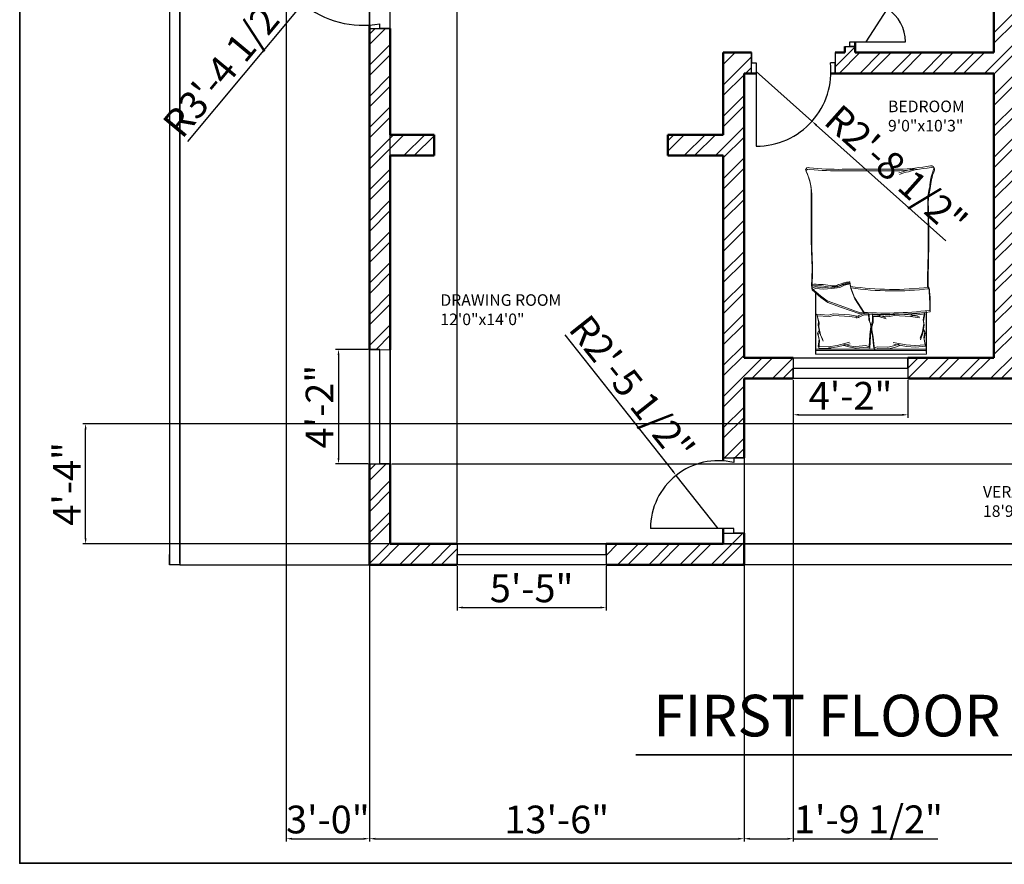
# Model space of a CAD drawing. Units: inches. Extents: x 1990 to 2869, y 1755 to 2533.
# Tile 1 of 6: x 1990 to 2415, y 1755 to 2120. Entities that reach past the tile are written whole.
import ezdxf

# ---------------------------------------------------------------- set-up
doc = ezdxf.new("R2010")
doc.units = ezdxf.units.IN
for name, color, linetype, lineweight in [('A-ANNO-DIMS', 171, 'Continuous', 18), ('A-ANNO-TTLB', 7, 'Continuous', 35), ('A-AREA-IDEN', 7, 'Continuous', 18), ('A-DOOR', 11, 'Continuous', 25), ('A-FLOR', 7, 'Continuous', 25), ('A-FURN', 8, 'Continuous', 18), ('A-GLAZ', 121, 'Continuous', 25), ('A-WALL', 7, 'Continuous', 50), ('A-WALL-SITE', 7, 'Continuous', 30)]:
    doc.layers.add(name, color=color, linetype=linetype, lineweight=lineweight)
doc.layers.add('A-WALL-PATT', color=215, linetype='Continuous', lineweight=13, true_color=0xa953a0)
doc.styles.get("Standard").update_dxf_attribs({"font": 'arial.ttf'})
doc.dimstyles.new('ISO-25', dxfattribs={"dimtxt": 12, "dimasz": 2.5, "dimexe": 1.25, "dimexo": 0.625, "dimtad": 1, "dimdec": 0, "dimlunit": 3, "dimtxsty": 'Standard', "dimcen": 2.5, "dimadec": 0, "dimazin": 0, "dimtfac": 1, "dimtdec": 0, "dimtmove": 0, "dimatfit": 3, "dimfxl": 1, "dimarcsym": 0})

# ---------------------------------------------------------------- blocks, each defined once
blk = doc.blocks.new('*D5')
at = {"layer": 'A-ANNO-DIMS', "color": 0, "lineweight": -2, "transparency": 16777216}
for p, q in [((2140.35, 1977.7), (2126.32, 1977.7)), ((2127.57, 1975.2), (2127.57, 1930.7)), ((2140.35, 1928.2), (2126.32, 1928.2))]:
    blk.add_line(p, q, dxfattribs=at)
at = {"layer": 'A-ANNO-DIMS', "color": 0, "transparency": 16777216}
for points in [[(2127.16, 1975.2), (2127.99, 1975.2), (2127.57, 1977.7)], [(2127.16, 1930.7), (2127.99, 1930.7), (2127.57, 1928.2)]]:
    blk.add_solid(points, dxfattribs=at)
at = {"layer": 'Defpoints', "color": 0, "transparency": 16777216}
for p in [(2140.97, 1977.7), (2127.57, 1928.2), (2140.97, 1928.2)]:
    blk.add_point(p, dxfattribs=at)
at = {"layer": 'A-ANNO-DIMS', "color": 0, "transparency": 16777216, "insert": (2120.92, 1952.95), "char_height": 12, "attachment_point": 5, "rotation": 90}
blk.add_mtext('4\'-2"', dxfattribs=at)
blk = doc.blocks.new('*D6')
at = {"layer": 'A-ANNO-DIMS', "color": 0, "lineweight": -2, "transparency": 16777216}
for p, q in [((2178.84, 1883.93), (2178.84, 1864.81)), ((2243.34, 1883.93), (2243.34, 1864.81)), ((2181.34, 1866.06), (2240.84, 1866.06))]:
    blk.add_line(p, q, dxfattribs=at)
at = {"layer": 'A-ANNO-DIMS', "color": 0, "transparency": 16777216}
for points in [[(2181.34, 1866.48), (2181.34, 1865.64), (2178.84, 1866.06)], [(2240.84, 1866.48), (2240.84, 1865.64), (2243.34, 1866.06)]]:
    blk.add_solid(points, dxfattribs=at)
at = {"layer": 'Defpoints', "color": 0, "transparency": 16777216}
for p in [(2178.84, 1884.55), (2243.34, 1884.55), (2243.34, 1866.06)]:
    blk.add_point(p, dxfattribs=at)
at = {"layer": 'A-ANNO-DIMS', "color": 0, "transparency": 16777216, "insert": (2211.09, 1872.79), "char_height": 12, "attachment_point": 5}
blk.add_mtext('5\'-5"', dxfattribs=at)
blk = doc.blocks.new('*D7')
at = {"layer": 'A-ANNO-DIMS', "color": 0, "lineweight": -2, "transparency": 16777216}
for p, q in [((2324.23, 1964.43), (2324.23, 1948.16)), ((2373.73, 1964.43), (2373.73, 1948.16)), ((2326.73, 1949.41), (2371.23, 1949.41))]:
    blk.add_line(p, q, dxfattribs=at)
at = {"layer": 'A-ANNO-DIMS', "color": 0, "transparency": 16777216}
for points in [[(2326.73, 1949.82), (2326.73, 1948.99), (2324.23, 1949.41)], [(2371.23, 1949.82), (2371.23, 1948.99), (2373.73, 1949.41)]]:
    blk.add_solid(points, dxfattribs=at)
at = {"layer": 'Defpoints', "color": 0, "transparency": 16777216}
for p in [(2324.23, 1965.05), (2373.73, 1965.05), (2373.73, 1949.41)]:
    blk.add_point(p, dxfattribs=at)
at = {"layer": 'A-ANNO-DIMS', "color": 0, "transparency": 16777216, "insert": (2348.98, 1956.06), "char_height": 12, "attachment_point": 5}
blk.add_mtext('4\'-2"', dxfattribs=at)
blk = doc.blocks.new('BED-DOUBLE')
for p, q in [((3.47, 63.33), (3.47, 81.44)), ((3.47, 81.44), (51.49, 81.44)), ((3.48, 63.33), (3.48, 81.44)), ((51.27, 81.44), (51.27, 54.83)), ((51.27, 81.44), (51.27, 54.83)), ((51.49, 81.44), (51.49, 80.8)), ((3.47, 79.91), (51.27, 79.91)), ((3.48, 79.91), (51.27, 79.91)), ((3.7, 62.69), (3.7, 80.8)), ((3.7, 62.69), (3.7, 80.8)), ((3.7, 79.27), (51.49, 79.27)), ((3.7, 79.27), (51.49, 79.27)), ((3.89, 78.13), (4.47, 74.95)), ((3.89, 78.13), (4.47, 74.95)), ((3.9, 78.11), (8.18, 78.43)), ((3.9, 78.11), (8.18, 78.43)), ((4.12, 77.49), (4.7, 74.31)), ((4.12, 77.49), (4.7, 74.31)), ((4.13, 77.47), (8.41, 77.8)), ((4.13, 77.47), (8.41, 77.8)), ((8.18, 78.43), (8.28, 78.42)), ((8.18, 78.43), (8.28, 78.42)), ((8.28, 78.42), (12.11, 78.13)), ((8.28, 78.42), (12.11, 78.13)), ((8.41, 77.8), (8.51, 77.78)), ((8.41, 77.8), (8.51, 77.78)), ((8.51, 77.78), (12.34, 77.49)), ((8.51, 77.78), (12.34, 77.49)), ((12.11, 78.13), (17.6, 77.11)), ((12.11, 78.13), (17.6, 77.11)), ((12.34, 77.49), (17.83, 76.48)), ((12.34, 77.49), (17.83, 76.48)), ((14.85, 77.69), (16.88, 78.42)), ((14.85, 77.69), (16.88, 78.42)), ((15.08, 77.05), (17.11, 77.78)), ((15.08, 77.05), (17.11, 77.78)), ((16.88, 78.42), (19.77, 79.14)), ((16.88, 78.42), (19.77, 79.14)), ((17.11, 77.78), (20, 78.5)), ((17.11, 77.78), (20, 78.5)), ((19.77, 79.14), (20.09, 79.14)), ((19.77, 79.14), (20.09, 79.14)), ((20, 78.5), (20.32, 78.5)), ((20, 78.5), (20.32, 78.5)), ((20.09, 79.14), (24.54, 78.99)), ((20.09, 79.14), (24.54, 78.99)), ((20.32, 78.5), (24.77, 78.36)), ((20.32, 78.5), (24.77, 78.36)), ((24.54, 78.99), (25.98, 79.57)), ((24.54, 78.99), (25.98, 79.57)), ((24.77, 78.36), (26.21, 78.93)), ((24.77, 78.36), (26.21, 78.93)), ((25.98, 79.57), (26.56, 74.22)), ((25.98, 79.57), (26.56, 74.22)), ((26.21, 78.93), (26.79, 73.58)), ((26.21, 78.93), (26.79, 73.58)), ((27.98, 78.95), (27.73, 73.58)), ((27.98, 78.95), (27.73, 73.58)), ((28.21, 78.31), (27.96, 72.94)), ((28.2, 78.31), (27.96, 72.94)), ((29.46, 78.46), (27.98, 78.95)), ((29.46, 78.46), (27.98, 78.95)), ((29.68, 77.82), (28.2, 78.31)), ((29.68, 77.82), (28.21, 78.31)), ((33.88, 78.89), (29.46, 78.46)), ((33.88, 78.89), (29.46, 78.46)), ((34.11, 78.25), (29.68, 77.82)), ((34.11, 78.25), (29.68, 77.82)), ((34.2, 78.91), (33.88, 78.89)), ((34.2, 78.91), (33.88, 78.89)), ((34.43, 78.27), (34.11, 78.25)), ((34.43, 78.27), (34.11, 78.25)), ((37.14, 78.36), (34.2, 78.91)), ((37.13, 78.36), (34.2, 78.91)), ((37.36, 77.73), (34.43, 78.27)), ((37.36, 77.73), (34.43, 78.27)), ((41.91, 78.37), (36.49, 77.02)), ((41.91, 78.37), (36.49, 77.02)), ((42.14, 77.73), (36.72, 76.38)), ((42.14, 77.73), (36.72, 76.38)), ((39.2, 77.77), (37.13, 78.36)), ((39.2, 77.77), (37.14, 78.36)), ((39.43, 77.13), (37.36, 77.73)), ((39.43, 77.13), (37.36, 77.73)), ((45.71, 78.9), (41.91, 78.37)), ((45.71, 78.9), (41.91, 78.37)), ((45.94, 78.26), (42.14, 77.73)), ((45.94, 78.26), (42.14, 77.73)), ((50.11, 78.89), (44.71, 78.98)), ((44.71, 78.98), (45.71, 78.9)), ((50.11, 78.89), (44.71, 78.98)), ((44.71, 78.98), (45.71, 78.9)), ((50.34, 78.25), (44.94, 78.34)), ((44.94, 78.34), (45.94, 78.26)), ((50.34, 78.25), (44.94, 78.34)), ((44.94, 78.34), (45.94, 78.26)), ((50.11, 78.89), (49.73, 75.68)), ((50.11, 78.89), (49.73, 75.68)), ((50.34, 78.25), (49.96, 75.04)), ((50.34, 78.25), (49.96, 75.04)), ((51.49, 80.8), (51.49, 54.19)), ((51.49, 80.8), (51.49, 54.19)), ((4.47, 74.95), (4.04, 72.34)), ((4.47, 74.95), (4.04, 72.34)), ((4.7, 74.31), (4.27, 71.7)), ((4.7, 74.31), (4.27, 71.7)), ((4.47, 68.87), (5.05, 72.49)), ((4.47, 68.87), (5.05, 72.49)), ((5.05, 72.49), (6.06, 75.24)), ((5.05, 72.49), (6.06, 75.24)), ((5.28, 71.85), (6.29, 74.6)), ((5.28, 71.85), (6.29, 74.6)), ((26.56, 74.22), (27.14, 71.04)), ((26.56, 74.22), (27.14, 71.04)), ((26.79, 73.58), (27.37, 70.4)), ((26.79, 73.58), (27.37, 70.4)), ((27.73, 73.58), (27.35, 70.37)), ((27.73, 73.58), (27.35, 70.37)), ((27.96, 72.94), (27.58, 69.73)), ((27.96, 72.94), (27.58, 69.73)), ((49.31, 73.19), (48.13, 75.86)), ((49.31, 73.19), (48.13, 75.86)), ((49.54, 72.55), (48.36, 75.23)), ((49.54, 72.55), (48.36, 75.23)), ((50.11, 69.61), (49.31, 73.19)), ((50.11, 69.61), (49.31, 73.19)), ((50.34, 68.98), (49.54, 72.55)), ((50.34, 68.98), (49.54, 72.55)), ((49.73, 75.68), (50.33, 73.1)), ((49.73, 75.68), (50.33, 73.1)), ((50.33, 73.1), (49.81, 72.06)), ((50.33, 73.1), (49.81, 72.06)), ((49.96, 75.04), (50.56, 72.47)), ((49.96, 75.04), (50.56, 72.47)), ((50.56, 72.47), (50.04, 71.42)), ((50.56, 72.47), (50.04, 71.42)), ((4.04, 72.34), (4.62, 71.33)), ((4.04, 72.34), (4.62, 71.33)), ((4.27, 71.7), (4.85, 70.69)), ((4.27, 71.7), (4.85, 70.69)), ((4.76, 67.28), (4.47, 68.87)), ((4.76, 67.28), (4.47, 68.87)), ((4.7, 68.23), (5.28, 71.85)), ((4.7, 68.23), (5.28, 71.85)), ((4.99, 66.64), (4.7, 68.23)), ((4.99, 66.64), (4.7, 68.23)), ((27.14, 69.74), (26.56, 67.86)), ((27.14, 69.74), (26.56, 67.86)), ((27.37, 69.1), (26.79, 67.22)), ((27.37, 69.1), (26.79, 67.22)), ((27.14, 71.04), (27.14, 69.74)), ((27.14, 71.04), (27.14, 69.74)), ((27.35, 70.37), (27.44, 69.07)), ((27.35, 70.37), (27.44, 69.07)), ((27.37, 70.4), (27.37, 69.1)), ((27.37, 70.4), (27.37, 69.1)), ((27.44, 69.07), (28.13, 67.23)), ((27.44, 69.07), (28.13, 67.23)), ((27.58, 69.73), (27.66, 68.43)), ((27.58, 69.73), (27.66, 68.43)), ((27.66, 68.43), (28.36, 66.59)), ((27.66, 68.43), (28.36, 66.59)), ((49.92, 68.01), (50.11, 69.61)), ((49.92, 68.01), (50.11, 69.61)), ((50.15, 67.37), (50.34, 68.98)), ((50.15, 67.37), (50.34, 68.98)), ((4.18, 64.1), (4.76, 67.28)), ((4.18, 64.1), (4.76, 67.28)), ((9.28, 64.82), (4.18, 64.1)), ((9.28, 64.82), (4.18, 64.1)), ((4.41, 63.46), (4.99, 66.64)), ((4.41, 63.46), (4.99, 66.64)), ((9.51, 64.19), (4.41, 63.46)), ((9.51, 64.19), (4.41, 63.46)), ((6.38, 65.81), (10.41, 65.15)), ((6.38, 65.81), (10.41, 65.15)), ((6.61, 65.18), (10.64, 64.51)), ((6.61, 65.18), (10.64, 64.51)), ((10.41, 65.15), (9.28, 64.82)), ((10.41, 65.15), (9.28, 64.82)), ((10.64, 64.51), (9.51, 64.19)), ((10.64, 64.51), (9.51, 64.19)), ((10.41, 65.15), (17.42, 64.72)), ((10.41, 65.15), (17.42, 64.72)), ((10.64, 64.51), (17.65, 64.08)), ((10.64, 64.51), (17.65, 64.08)), ((17.42, 64.72), (19.38, 65.27)), ((17.42, 64.72), (19.38, 65.27)), ((17.65, 64.08), (19.61, 64.63)), ((17.65, 64.08), (19.61, 64.63)), ((19.38, 65.27), (24.52, 64.87)), ((19.38, 65.27), (24.52, 64.87)), ((19.61, 64.63), (24.74, 64.23)), ((19.61, 64.63), (24.74, 64.23)), ((24.1, 65.18), (20.96, 66.27)), ((24.1, 65.18), (20.96, 66.27)), ((24.33, 64.54), (21.19, 65.63)), ((24.33, 64.54), (21.19, 65.63)), ((26.56, 65.18), (24.1, 65.18)), ((26.56, 65.18), (24.1, 65.18)), ((26.79, 64.54), (24.33, 64.54)), ((26.79, 64.54), (24.33, 64.54)), ((26.56, 67.86), (26.56, 65.18)), ((26.56, 67.86), (26.56, 65.18)), ((26.79, 67.22), (26.79, 64.54)), ((26.79, 67.22), (26.79, 64.54)), ((28.13, 67.23), (28.3, 64.55)), ((28.13, 67.23), (28.3, 64.55)), ((28.3, 64.55), (30.75, 64.7)), ((28.3, 64.55), (30.75, 64.7)), ((28.36, 66.59), (28.53, 63.91)), ((28.36, 66.59), (28.53, 63.91)), ((28.53, 63.91), (30.98, 64.06)), ((28.53, 63.91), (30.98, 64.06)), ((30.26, 64.06), (34.45, 57.57)), ((30.26, 64.06), (34.45, 57.57)), ((30.75, 64.7), (33.82, 65.99)), ((30.75, 64.7), (33.82, 65.99)), ((30.98, 64.06), (34.05, 65.35)), ((30.98, 64.06), (34.05, 65.35)), ((40.64, 61.13), (32.31, 64.06)), ((40.64, 61.13), (32.31, 64.06)), ((32.56, 65.81), (36.6, 65.15)), ((32.56, 65.81), (36.6, 65.15)), ((32.79, 65.18), (36.82, 64.51)), ((32.79, 65.18), (36.82, 64.51)), ((36.6, 65.15), (43.61, 64.72)), ((36.6, 65.15), (43.61, 64.72)), ((36.82, 64.51), (43.83, 64.08)), ((36.82, 64.51), (43.83, 64.08)), ((43.61, 64.72), (45.57, 65.27)), ((43.61, 64.72), (45.57, 65.27)), ((43.83, 64.08), (45.79, 64.63)), ((43.83, 64.08), (45.79, 64.63)), ((45.57, 65.27), (50.7, 64.87)), ((45.57, 65.27), (50.7, 64.87)), ((45.79, 64.63), (50.93, 64.23)), ((45.79, 64.63), (50.93, 64.23)), ((50.7, 64.87), (49.92, 68.01)), ((50.7, 64.87), (49.92, 68.01)), ((50.93, 64.23), (50.15, 67.37)), ((50.93, 64.23), (50.15, 67.37)), ((30.49, 63.42), (34.68, 56.93)), ((30.49, 63.42), (34.68, 56.93)), ((40.87, 60.49), (32.53, 63.42)), ((40.87, 60.49), (32.53, 63.42)), ((46.22, 59.11), (40.64, 61.13)), ((46.22, 59.11), (40.64, 61.13)), ((46.45, 58.48), (40.87, 60.49)), ((46.45, 58.48), (40.87, 60.49)), ((34.45, 57.57), (36.15, 53.08)), ((34.45, 57.57), (36.15, 53.08)), ((34.68, 56.93), (36.38, 52.44)), ((34.68, 56.93), (36.38, 52.44)), ((49.16, 56.95), (46.22, 59.11)), ((49.16, 56.95), (46.22, 59.11)), ((49.39, 56.31), (46.45, 58.48)), ((49.39, 56.31), (46.45, 58.48)), ((52.87, 53.7), (49.16, 56.95)), ((52.87, 53.7), (49.16, 56.95)), ((53.1, 53.06), (49.39, 56.31)), ((53.1, 53.06), (49.39, 56.31)), ((36.15, 53.08), (36.46, 51.07)), ((36.15, 53.08), (36.46, 51.07)), ((36.38, 52.44), (36.69, 50.43)), ((36.38, 52.44), (36.69, 50.43)), ((36.46, 51.07), (38.94, 51.69)), ((36.46, 51.07), (38.94, 51.69)), ((38.94, 51.69), (40.95, 52.61)), ((38.94, 51.69), (40.95, 52.61)), ((39.17, 51.05), (41.18, 51.97)), ((39.17, 51.05), (41.18, 51.97)), ((40.95, 52.61), (44.36, 53.08)), ((40.95, 52.61), (44.36, 53.08)), ((41.18, 51.97), (44.59, 52.44)), ((41.18, 51.97), (44.59, 52.44)), ((44.36, 53.08), (48.23, 53.39)), ((44.36, 53.08), (48.23, 53.39)), ((44.59, 52.44), (48.46, 52.75)), ((44.59, 52.44), (48.46, 52.75)), ((48.23, 53.39), (51.33, 53.08)), ((48.23, 53.39), (51.33, 53.08)), ((48.46, 52.75), (51.56, 52.44)), ((48.46, 52.75), (51.56, 52.44)), ((51.33, 53.08), (52.87, 53.7)), ((51.33, 53.08), (52.87, 53.7)), ((51.56, 52.44), (53.1, 53.06)), ((51.56, 52.44), (53.1, 53.06)), ((52.95, 51.95), (52.87, 53.7, 3.87)), ((52.95, 51.95), (52.87, 53.7, 3.87)), ((53.18, 51.31), (53.1, 53.06, 3.87)), ((53.18, 51.31), (53.1, 53.06, 3.87)), ((36.69, 50.43), (39.17, 51.05)), ((36.69, 50.43), (39.17, 51.05)), ((15.06, 2.2), (39.68, 2.2)), ((15.06, 2.2), (39.68, 2.2)), ((15.29, 1.56), (39.91, 1.56)), ((15.29, 1.56), (39.91, 1.56))]:
    blk.add_line(p, q)
for centre, radius, start, end in [((21.36, -100.61), 164.97, 86.0865, 96.7821), ((21.36, -100.61), 164.97, 86.0865, 96.7821), ((85.16, 61.35), 83.31, 178.7218, 185.604), ((85.16, 61.35), 83.31, 178.7218, 185.604), ((85.39, 60.71), 83.31, 178.7218, 185.604), ((85.39, 60.71), 83.31, 178.7218, 185.604), ((21.59, -101.25), 164.97, 86.0865, 96.7821), ((21.59, -101.25), 164.97, 86.0865, 96.7821), ((17.76, -74.87), 129.02, 81.7845, 96.9006), ((17.76, -74.87), 129.02, 81.7845, 96.9006), ((17.98, -75.51), 129.02, 81.7845, 96.9006), ((17.98, -75.51), 129.02, 81.7845, 96.9006), ((-167.31, 50.27), 170.11, 358.4762, 1.0082), ((-167.31, 50.27), 170.11, 358.4762, 1.0082), ((-167.08, 49.63), 170.11, 358.4762, 1.0082), ((-167.08, 49.63), 170.11, 358.4762, 1.0082), ((31.15, 79.96), 29.65, 280.6617, 289.8806), ((31.15, 79.96), 29.65, 280.6617, 289.8806), ((31.38, 79.32), 29.65, 280.6617, 289.8806), ((31.38, 79.32), 29.65, 280.6617, 289.8806), ((43.74, 46.38), 6.22, 78.6608, 113.7384), ((43.74, 46.38), 6.22, 78.6608, 113.7384), ((43.97, 45.74), 6.22, 78.6608, 113.7384), ((43.97, 45.74), 6.22, 78.6608, 113.7384), ((51.33, 88.1), 36.18, 259.8763, 272.5657), ((51.33, 88.1), 36.18, 259.8763, 272.5657), ((51.56, 87.46), 36.18, 259.8763, 272.5657), ((51.56, 87.46), 36.18, 259.8763, 272.5657), ((182.27, 45.13), 129.5, 176.9791, 183.8365), ((182.27, 45.13), 129.5, 176.9791, 183.8365), ((182.49, 44.49), 129.5, 176.9791, 183.8365), ((182.49, 44.49), 129.5, 176.9791, 183.8365), ((36.64, 51), 0.185, 160.2464, 271.1377), ((36.64, 51), 0.185, 160.2464, 271.1377), ((36.86, 50.36), 0.185, 160.2464, 271.1377), ((36.86, 50.36), 0.185, 160.2464, 271.1377), ((484.82, 30.83), 482.31, 178.2277, 181.7185), ((484.82, 30.83), 482.31, 178.2277, 181.7185), ((485.05, 30.19), 482.31, 178.2277, 181.7185), ((485.05, 30.19), 482.31, 178.2277, 181.7185), ((-4508.74, 13.62), 4561.86, 0.00217, 0.28689), ((-4508.74, 13.62), 4561.86, 0.00217, 0.28689), ((-4508.52, 12.98), 4561.86, 0.00217, 0.28689), ((-4508.52, 12.98), 4561.86, 0.00217, 0.28689), ((-26.9, 16.93), 29.63, 346.0648, 358.9113), ((-26.9, 16.93), 29.63, 346.0648, 358.9113), ((-26.67, 16.29), 29.63, 346.0648, 358.9113), ((-26.67, 16.29), 29.63, 346.0648, 358.9113), ((76.16, 12.78), 23.07, 177.4714, 206.4681), ((76.16, 12.78), 23.07, 177.4714, 206.4681), ((76.39, 12.14), 23.07, 177.4714, 206.4681), ((76.39, 12.14), 23.07, 177.4714, 206.4681), ((-21.66, 11.17), 23.56, 337.9751, 356.652), ((-21.66, 11.17), 23.56, 337.9751, 356.652), ((-21.43, 10.53), 23.56, 337.9751, 356.652), ((-21.43, 10.53), 23.56, 337.9751, 356.652), ((1.09, 1.73), 1.09, 146.1736, 293.4781), ((1.09, 1.73), 1.09, 146.1736, 293.4781), ((1.32, 1.09), 1.09, 146.1736, 293.4781), ((1.32, 1.09), 1.09, 146.1736, 293.4781), ((21.43, -119.39), 121.76, 92.9958, 99.4091), ((21.43, -119.39), 121.76, 92.9958, 99.4091), ((21.66, -120.03), 121.76, 92.9958, 99.4091), ((21.65, -120.03), 121.76, 92.9958, 99.4091), ((-17.22, 105.15), 106.46, 283.3832, 287.7053), ((-17.22, 105.15), 106.46, 283.3832, 287.7053), ((-16.99, 104.52), 106.46, 283.3832, 287.7053), ((-16.99, 104.52), 106.46, 283.3832, 287.7053), ((41.15, -130.83), 133.04, 84.4998, 90.6351), ((41.15, -130.83), 133.04, 84.4998, 90.6351), ((41.38, -131.47), 133.04, 84.4998, 90.6351), ((41.38, -131.47), 133.04, 84.4998, 90.6351), ((54.41, 2.57), 1.1, 242.6588, 356.02), ((54.41, 2.57), 1.1, 242.6588, 356.02), ((54.64, 1.93), 1.1, 242.6588, 356.02), ((54.64, 1.93), 1.1, 242.6588, 356.02)]:
    blk.add_arc(centre, radius, start, end)
blk = doc.blocks.new('WIN-49_5IN')
for p, q in [((0, 9), (0, 0)), ((0, 9), (49.5, 9)), ((49.5, 4.5), (49.5, 9)), ((49.5, 9), (49.5, 0)), ((0, 0), (0, 4.5)), ((0, 4.5), (49.5, 4.5)), ((49.5, 0), (0, 0))]:
    blk.add_line(p, q)
blk = doc.blocks.new('WIN-64_5IN')
for p, q in [((0, 9), (0, 0)), ((0, 9), (64.5, 9)), ((64.5, 4.5), (64.5, 9)), ((64.5, 9), (64.5, 0)), ((0, 0), (0, 4.5)), ((0, 4.5), (64.5, 4.5)), ((64.5, 0), (0, 0))]:
    blk.add_line(p, q)
blk = doc.blocks.new('*D23')
at = {"layer": 'A-ANNO-DIMS', "color": 0, "lineweight": -2, "transparency": 16777216}
for p, q in [((2435.03, 2169.19), (2437.82, 2169.19)), ((2436.57, 2166.69), (2436.57, 2161.95)), ((2435.03, 2159.45), (2437.82, 2159.45)), ((2436.57, 2159.45), (2436.57, 2054.59))]:
    blk.add_line(p, q, dxfattribs=at)
at = {"layer": 'A-ANNO-DIMS', "color": 0, "transparency": 16777216}
for points in [[(2436.15, 2166.69), (2436.99, 2166.69), (2436.57, 2169.19)], [(2436.15, 2161.95), (2436.99, 2161.95), (2436.57, 2159.45)]]:
    blk.add_solid(points, dxfattribs=at)
at = {"layer": 'Defpoints', "color": 0, "transparency": 16777216}
for p in [(2434.41, 2169.19), (2434.41, 2159.45), (2436.57, 2159.45)]:
    blk.add_point(p, dxfattribs=at)
at = {"layer": 'A-ANNO-DIMS', "color": 0, "transparency": 16777216, "insert": (2429.74, 2105.77), "char_height": 12, "attachment_point": 5, "rotation": 90}
blk.add_mtext('0\'-9 1/2" TYP.', dxfattribs=at)
blk = doc.blocks.new('*D24')
at = {"layer": 'A-ANNO-DIMS', "color": 0, "lineweight": -2, "transparency": 16777216}
for p, q in [((2149.97, 1894.18), (2149.97, 2365.55)), ((2152.47, 2364.3), (2176.34, 2364.3)), ((2178.84, 1894.18), (2178.84, 2365.55)), ((2178.84, 2364.3), (2214.69, 2364.3))]:
    blk.add_line(p, q, dxfattribs=at)
at = {"layer": 'A-ANNO-DIMS', "color": 0, "transparency": 16777216}
for points in [[(2152.47, 2364.72), (2152.47, 2363.88), (2149.97, 2364.3)], [(2176.34, 2364.72), (2176.34, 2363.88), (2178.84, 2364.3)]]:
    blk.add_solid(points, dxfattribs=at)
at = {"layer": 'Defpoints', "color": 0, "transparency": 16777216}
for p in [(2178.84, 2364.3), (2149.97, 1893.55), (2178.84, 1893.55)]:
    blk.add_point(p, dxfattribs=at)
at = {"layer": 'A-ANNO-DIMS', "color": 0, "transparency": 16777216, "insert": (2198.02, 2371.05), "char_height": 12, "attachment_point": 5}
blk.add_mtext('2\'-5"', dxfattribs=at)
blk = doc.blocks.new('*D25')
at = {"layer": 'A-ANNO-DIMS', "color": 0, "lineweight": -2, "transparency": 16777216}
for p, q in [((2058.97, 1885.18), (2058.97, 2365.55)), ((2061.47, 2364.3), (2138.47, 2364.3)), ((2140.97, 1885.18), (2140.97, 2365.55))]:
    blk.add_line(p, q, dxfattribs=at)
at = {"layer": 'A-ANNO-DIMS', "color": 0, "transparency": 16777216}
for points in [[(2061.47, 2364.72), (2061.47, 2363.88), (2058.97, 2364.3)], [(2138.47, 2364.72), (2138.47, 2363.88), (2140.97, 2364.3)]]:
    blk.add_solid(points, dxfattribs=at)
at = {"layer": 'Defpoints', "color": 0, "transparency": 16777216}
for p in [(2140.97, 2364.3), (2058.97, 1884.55), (2140.97, 1884.55)]:
    blk.add_point(p, dxfattribs=at)
at = {"layer": 'A-ANNO-DIMS', "color": 0, "transparency": 16777216, "insert": (2099.97, 2371.05), "char_height": 12, "attachment_point": 5}
blk.add_mtext('6\'-10"', dxfattribs=at)
blk = doc.blocks.new('*D26')
at = {"layer": 'A-ANNO-DIMS', "color": 0, "lineweight": -2, "transparency": 16777216}
for p, q in [((2140.97, 1883.93), (2140.97, 1764.83)), ((2302.97, 1883.93), (2302.97, 1764.83)), ((2143.47, 1766.08), (2300.47, 1766.08))]:
    blk.add_line(p, q, dxfattribs=at)
at = {"layer": 'A-ANNO-DIMS', "color": 0, "transparency": 16777216}
for points in [[(2143.47, 1766.49), (2143.47, 1765.66), (2140.97, 1766.08)], [(2300.47, 1766.49), (2300.47, 1765.66), (2302.97, 1766.08)]]:
    blk.add_solid(points, dxfattribs=at)
at = {"layer": 'Defpoints', "color": 0, "transparency": 16777216}
for p in [(2140.97, 1884.55), (2302.97, 1884.55), (2302.97, 1766.08)]:
    blk.add_point(p, dxfattribs=at)
at = {"layer": 'A-ANNO-DIMS', "color": 0, "transparency": 16777216, "insert": (2221.97, 1772.83), "char_height": 12, "attachment_point": 5}
blk.add_mtext('13\'-6"', dxfattribs=at)
blk = doc.blocks.new('*D28')
at = {"layer": 'A-ANNO-DIMS', "color": 0, "lineweight": -2, "transparency": 16777216}
for p, q in [((2812.72, 1928.2), (2812.72, 2001.34)), ((2150.6, 1928.2), (2813.97, 1928.2)), ((2812.72, 1896.05), (2812.72, 1925.7)), ((2150.6, 1893.55), (2813.97, 1893.55))]:
    blk.add_line(p, q, dxfattribs=at)
at = {"layer": 'A-ANNO-DIMS', "color": 0, "transparency": 16777216}
for points in [[(2812.3, 1925.7), (2813.14, 1925.7), (2812.72, 1928.2)], [(2812.3, 1896.05), (2813.14, 1896.05), (2812.72, 1893.55)]]:
    blk.add_solid(points, dxfattribs=at)
at = {"layer": 'Defpoints', "color": 0, "transparency": 16777216}
for p in [(2149.97, 1928.2), (2812.72, 1928.2), (2149.97, 1893.55)]:
    blk.add_point(p, dxfattribs=at)
at = {"layer": 'A-ANNO-DIMS', "color": 0, "transparency": 16777216, "insert": (2805.89, 1966.02), "char_height": 12, "attachment_point": 5, "rotation": 90}
blk.add_mtext('2\'-10 1/2"', dxfattribs=at)
blk = doc.blocks.new('*D29')
at = {"layer": 'A-ANNO-DIMS', "color": 0, "lineweight": -2, "transparency": 16777216}
for p, q in [((2680.35, 1945.55), (2016.97, 1945.55)), ((2018.22, 1896.05), (2018.22, 1943.05)), ((2680.35, 1893.55), (2016.97, 1893.55))]:
    blk.add_line(p, q, dxfattribs=at)
at = {"layer": 'A-ANNO-DIMS', "color": 0, "transparency": 16777216}
for points in [[(2017.8, 1943.05), (2018.64, 1943.05), (2018.22, 1945.55)], [(2017.8, 1896.05), (2018.64, 1896.05), (2018.22, 1893.55)]]:
    blk.add_solid(points, dxfattribs=at)
at = {"layer": 'Defpoints', "color": 0, "transparency": 16777216}
for p in [(2018.22, 1945.55), (2680.97, 1945.55), (2680.97, 1893.55)]:
    blk.add_point(p, dxfattribs=at)
at = {"layer": 'A-ANNO-DIMS', "color": 0, "transparency": 16777216, "insert": (2011.6, 1919.55), "char_height": 12, "attachment_point": 5, "rotation": 90}
blk.add_mtext('4\'-4"', dxfattribs=at)
blk = doc.blocks.new('*D31')
at = {"layer": 'A-ANNO-DIMS', "color": 0, "lineweight": -2, "transparency": 16777216}
for p, q in [((2302.97, 1964.43), (2302.97, 1764.83)), ((2324.23, 1964.43), (2324.23, 1764.83)), ((2305.47, 1766.08), (2321.73, 1766.08)), ((2324.23, 1766.08), (2386.71, 1766.08))]:
    blk.add_line(p, q, dxfattribs=at)
at = {"layer": 'A-ANNO-DIMS', "color": 0, "transparency": 16777216}
for points in [[(2305.47, 1766.49), (2305.47, 1765.66), (2302.97, 1766.08)], [(2321.73, 1766.49), (2321.73, 1765.66), (2324.23, 1766.08)]]:
    blk.add_solid(points, dxfattribs=at)
at = {"layer": 'Defpoints', "color": 0, "transparency": 16777216}
for p in [(2302.97, 1965.05), (2324.23, 1965.05), (2324.23, 1766.08)]:
    blk.add_point(p, dxfattribs=at)
at = {"layer": 'A-ANNO-DIMS', "color": 0, "transparency": 16777216, "insert": (2356.72, 1772.91), "char_height": 12, "attachment_point": 5}
blk.add_mtext('1\'-9 1/2"', dxfattribs=at)
blk = doc.blocks.new('*D33')
at = {"layer": 'A-ANNO-DIMS', "color": 0, "lineweight": -2, "transparency": 16777216}
for p, q in [((2104.97, 2165.93), (2104.97, 1764.83)), ((2140.97, 2165.93), (2140.97, 1764.83)), ((2107.47, 1766.08), (2138.47, 1766.08))]:
    blk.add_line(p, q, dxfattribs=at)
at = {"layer": 'A-ANNO-DIMS', "color": 0, "transparency": 16777216}
for points in [[(2107.47, 1766.49), (2107.47, 1765.66), (2104.97, 1766.08)], [(2138.47, 1766.49), (2138.47, 1765.66), (2140.97, 1766.08)]]:
    blk.add_solid(points, dxfattribs=at)
at = {"layer": 'Defpoints', "color": 0, "transparency": 16777216}
for p in [(2104.97, 2166.55), (2140.97, 2166.55), (2140.97, 1766.08)]:
    blk.add_point(p, dxfattribs=at)
at = {"layer": 'A-ANNO-DIMS', "color": 0, "transparency": 16777216, "insert": (2122.97, 1772.83), "char_height": 12, "attachment_point": 5}
blk.add_mtext('3\'-0"', dxfattribs=at)
blk = doc.blocks.new('*D50')
at = {"layer": 'A-ANNO-DIMS', "color": 0, "lineweight": -2, "transparency": 16777216}
for p, q in [((2138.1, 2158.48), (2112.11, 2127.26)), ((2062.46, 2067.62), (2110.51, 2125.33))]:
    blk.add_line(p, q, dxfattribs=at)
at = {"layer": 'A-ANNO-DIMS', "color": 0, "transparency": 16777216}
blk.add_solid([(2110.19, 2125.6), (2110.83, 2125.07), (2112.11, 2127.26)], dxfattribs=at)
at = {"layer": 'Defpoints', "color": 0, "transparency": 16777216}
for p in [(2138.1, 2158.48), (2112.11, 2127.26)]:
    blk.add_point(p, dxfattribs=at)
at = {"layer": 'A-ANNO-DIMS', "color": 0, "transparency": 16777216, "insert": (2080.43, 2099.89), "char_height": 12, "attachment_point": 5, "rotation": 50.2228}
blk.add_mtext('R3\'-4 1/2"', dxfattribs=at)
blk = doc.blocks.new('*D52')
at = {"layer": 'A-ANNO-DIMS', "color": 0, "lineweight": -2, "transparency": 16777216}
for p, q in [((2225.37, 1984.01), (2272.02, 1925.17)), ((2291.79, 1900.24), (2273.57, 1923.21))]:
    blk.add_line(p, q, dxfattribs=at)
at = {"layer": 'A-ANNO-DIMS', "color": 0, "transparency": 16777216}
blk.add_solid([(2272.35, 1925.43), (2271.69, 1924.91), (2273.57, 1923.21)], dxfattribs=at)
at = {"layer": 'Defpoints', "color": 0, "transparency": 16777216}
for p in [(2273.57, 1923.21), (2291.79, 1900.24)]:
    blk.add_point(p, dxfattribs=at)
at = {"layer": 'A-ANNO-DIMS', "color": 0, "transparency": 16777216, "insert": (2253.27, 1959.81), "char_height": 12, "attachment_point": 5, "rotation": 308.4096}
blk.add_mtext('R2\'-5 1/2"', dxfattribs=at)
blk = doc.blocks.new('*D57')
at = {"layer": 'A-ANNO-DIMS', "color": 0, "lineweight": -2, "transparency": 16777216}
for p, q in [((2308.2, 2097.87), (2332.31, 2076.36)), ((2390.23, 2024.71), (2334.18, 2074.69))]:
    blk.add_line(p, q, dxfattribs=at)
at = {"layer": 'A-ANNO-DIMS', "color": 0, "transparency": 16777216}
blk.add_solid([(2334.46, 2075.01), (2333.9, 2074.38), (2332.31, 2076.36)], dxfattribs=at)
at = {"layer": 'Defpoints', "color": 0, "transparency": 16777216}
for p in [(2308.2, 2097.87), (2332.31, 2076.36)]:
    blk.add_point(p, dxfattribs=at)
at = {"layer": 'A-ANNO-DIMS', "color": 0, "transparency": 16777216, "insert": (2367.68, 2053.97), "char_height": 12, "attachment_point": 5, "rotation": 318.2723}
blk.add_mtext('R2\'-8 1/2"', dxfattribs=at)
blk = doc.blocks.new('*D61')
at = {"layer": 'A-ANNO-DIMS', "color": 0, "lineweight": -2, "transparency": 16777216}
for p, q in [((2391.86, 2166.71), (2366.3, 2127.11)), ((2355.72, 2110.72), (2364.94, 2125.01))]:
    blk.add_line(p, q, dxfattribs=at)
at = {"layer": 'A-ANNO-DIMS', "color": 0, "transparency": 16777216}
blk.add_solid([(2365.95, 2127.34), (2366.65, 2126.88), (2364.94, 2125.01)], dxfattribs=at)
at = {"layer": 'Defpoints', "color": 0, "transparency": 16777216}
for p in [(2364.94, 2125.01), (2355.72, 2110.72)]:
    blk.add_point(p, dxfattribs=at)
at = {"layer": 'A-ANNO-DIMS', "color": 0, "transparency": 16777216, "insert": (2374.09, 2151.62), "char_height": 12, "attachment_point": 5, "rotation": 57.1524}
blk.add_mtext('R1\'-5"', dxfattribs=at)

msp = doc.modelspace()

# ---------------------------------------------------------------- hatches: boundary and pattern name
at = {"layer": 'A-WALL-PATT'}
h = msp.add_hatch(dxfattribs=at)
h.set_pattern_fill('ANSI32', color=256)
h.paths.add_polyline_path([(2193.46, 2287.55), (2131.97, 2287.55), (2131.97, 2278.55), (2193.46, 2278.55)])
h.paths.add_polyline_path([(2113.97, 2278.55), (2113.97, 2287.55), (2104.97, 2287.55), (2104.97, 2257.5), (2113.97, 2257.5)])
h.paths.add_polyline_path([(2113.97, 2205), (2104.97, 2205), (2104.97, 2166.55), (2140.97, 2166.55), (2140.97, 2160.48), (2149.97, 2160.48), (2149.97, 2166.55), (2170.14, 2166.55), (2170.14, 2175.55), (2113.97, 2175.55)])
h.paths.add_polyline_path([(2278.97, 2287.55), (2244.47, 2287.55), (2244.47, 2278.55), (2274.47, 2278.55), (2274.47, 2200.55), (2226.47, 2200.55), (2226.47, 2219.37), (2221.97, 2219.37), (2221.97, 2175.55), (2221.97, 2166.55), (2226.47, 2166.55), (2226.47, 2196.05), (2274.47, 2196.05), (2274.47, 2166.55), (2284.01, 2166.55), (2284.01, 2171.05), (2284.01, 2175.55), (2278.97, 2175.55), (2278.97, 2278.55)])
h.paths.add_polyline_path([(2226.47, 2283.05), (2226.47, 2287.55), (2217.66, 2287.55), (2217.66, 2283.05), (2217.66, 2278.55), (2221.97, 2278.55), (2221.97, 2255.21), (2226.47, 2255.21), (2226.47, 2278.55)])
h.paths.add_polyline_path([(2560.97, 2328.05), (2551.97, 2328.05), (2269.97, 2328.05), (2269.97, 2319.05), (2278.97, 2319.05), (2410.97, 2319.05), (2410.97, 2187.05), (2346.47, 2187.05), (2346.47, 2175.55), (2319.77, 2175.55), (2319.77, 2166.55), (2346.47, 2166.55), (2346.47, 2128.22), (2350.97, 2128.22), (2350.97, 2178.05), (2410.97, 2178.05), (2410.97, 2175.55), (2410.97, 2106.05), (2350.97, 2106.05), (2350.97, 2108.72), (2348.72, 2108.72), (2346.47, 2108.72), (2346.47, 2106.05), (2342.3, 2106.05), (2342.3, 2097.05), (2346.47, 2097.05), (2350.97, 2097.05), (2410.97, 2097.05), (2410.97, 1974.05), (2373.73, 1974.05), (2373.73, 1965.05), (2419.97, 1965.05), (2447.99, 1965.05), (2447.99, 1969.55), (2447.99, 1974.05), (2419.97, 1974.05), (2419.97, 2097.05), (2484.47, 2097.05), (2489.55, 2097.05), (2489.55, 2106.05), (2484.47, 2106.05), (2484.47, 2108.84), (2482.22, 2108.84), (2479.97, 2108.84), (2479.97, 2106.05), (2419.97, 2106.05), (2419.97, 2175.55), (2419.97, 2178.05), (2479.97, 2178.05), (2479.97, 2128.49), (2484.47, 2128.49), (2484.47, 2166.55), (2511.88, 2166.55), (2511.88, 2171.05), (2511.88, 2175.55), (2484.47, 2175.55), (2484.47, 2187.05), (2479.97, 2187.05), (2419.97, 2187.05), (2419.97, 2319.05), (2551.97, 2319.05), (2560.97, 2319.05)])
h.paths.add_polyline_path([(2586.47, 2292.05), (2560.97, 2292.05), (2551.97, 2292.05), (2551.97, 2175.55), (2547.37, 2175.55), (2547.37, 2166.55), (2556.47, 2166.55), (2556.47, 2175.55), (2556.47, 2205.05), (2604.47, 2205.05), (2604.47, 2166.55), (2608.97, 2166.55), (2608.97, 2175.55), (2608.97, 2205.05), (2608.97, 2228.1), (2604.47, 2228.1), (2604.47, 2209.55), (2556.47, 2209.55), (2556.47, 2283.05), (2586.47, 2283.05)])
h.paths.add_polyline_path([(2691.55, 2292.05), (2690.86, 2292.05), (2636.82, 2292.05), (2636.82, 2283.05), (2691.55, 2283.05)])
h.paths.add_polyline_path([(2725.97, 2292.05), (2716.97, 2292.05), (2709.55, 2292.05), (2709.55, 2287.55), (2709.55, 2283.05), (2716.97, 2283.05), (2716.97, 2263.68), (2725.97, 2263.68)])
h.paths.add_polyline_path([(2725.97, 2199.18), (2716.97, 2199.18), (2716.97, 2180.05), (2716.97, 2175.55), (2650.43, 2175.55), (2650.43, 2166.55), (2680.97, 2166.55), (2680.97, 2159.77), (2689.97, 2159.77), (2689.97, 2166.55), (2725.97, 2166.55)])
h.paths.add_polyline_path([(2536.97, 2061.55), (2554.82, 2061.55), (2554.82, 2070.55), (2536.97, 2070.55), (2536.97, 2097.05), (2536.97, 2106.05), (2524.42, 2106.05), (2524.42, 2101.55), (2524.42, 2097.05), (2527.97, 2097.05), (2527.97, 1974.05), (2497.49, 1974.05), (2497.49, 1965.05), (2527.97, 1965.05), (2527.97, 1929.96), (2536.97, 1929.96)])
h.paths.add_polyline_path([(2689.97, 1945.55), (2685.47, 1945.55), (2680.97, 1945.55), (2680.97, 1893.55), (2625.68, 1893.55), (2625.68, 1884.55), (2689.97, 1884.55), (2689.97, 1893.55)])
h.paths.add_polyline_path([(2168.89, 2070.55), (2149.97, 2070.55), (2149.97, 2116.52), (2145.47, 2116.52), (2140.97, 2116.52), (2140.97, 1977.7), (2145.47, 1977.7), (2145.47, 1977.63), (2149.97, 1977.55), (2149.97, 2061.55), (2168.89, 2061.55)])
h.paths.add_polyline_path([(2302.97, 2097.05), (2306.2, 2097.05), (2306.2, 2106.05), (2293.97, 2106.05), (2293.97, 2097.05), (2293.97, 2070.55), (2269.93, 2070.55), (2269.93, 2061.55), (2293.97, 2061.55), (2293.97, 1930.78), (2302.97, 1930.78), (2302.97, 1965.05), (2324.23, 1965.05), (2324.23, 1969.55), (2324.23, 1974.05), (2302.97, 1974.05)])
h.paths.add_polyline_path([(2149.97, 1928.2), (2145.47, 1928.2), (2140.97, 1928.2), (2140.97, 1889.05), (2140.97, 1884.55), (2178.84, 1884.55), (2178.84, 1889.05), (2178.84, 1893.55), (2149.97, 1893.55)])
h.paths.add_polyline_path([(2302.97, 1898.24), (2298.47, 1898.24), (2293.97, 1898.24), (2293.97, 1893.55), (2243.34, 1893.55), (2243.34, 1884.55), (2302.97, 1884.55)])

# ---------------------------------------------------------------- linework, layer by layer
at = {"layer": 'A-ANNO-TTLB'}
msp.add_line((2256.16, 1802.33), (2506.84, 1802.33), dxfattribs=at)
msp.add_lwpolyline([(1989.71, 2378.83), (2869.46, 2378.83), (2869.46, 1755.45), (1989.71, 1755.45)], close=True, dxfattribs=at)
at = {"layer": 'A-DOOR'}
for p, q in [((2140.97, 2116.52), (2149.97, 2116.52)), ((2145.47, 2116.52), (2145.47, 2118.52)), ((2149.97, 2116.52), (2145.47, 2116.52)), ((2346.47, 2108.72), (2350.97, 2108.72)), ((2348.72, 2108.72), (2348.72, 2110.72)), ((2348.72, 2110.72), (2372.72, 2110.72)), ((2350.97, 2108.72), (2348.72, 2108.72)), ((2306.2, 2097.05), (2306.2, 2106.05)), ((2306.2, 2106.05), (2306.2, 2101.55)), ((2342.3, 2106.05), (2342.3, 2097.05)), ((2306.2, 2101.55), (2308.2, 2101.55)), ((2308.2, 2101.55), (2308.2, 2065.55)), ((2342.3, 2101.55), (2340.3, 2101.55)), ((2342.3, 2097.05), (2342.3, 2101.55)), ((2293.97, 1930.78), (2302.97, 1930.78)), ((2302.97, 1930.78), (2298.47, 1930.78)), ((2298.47, 1930.78), (2298.47, 1928.78)), ((2298.47, 1900.24), (2262.47, 1900.24)), ((2298.47, 1898.24), (2298.47, 1900.24)), ((2293.97, 1898.24), (2302.97, 1898.24)), ((2302.97, 1898.24), (2298.47, 1898.24))]:
    msp.add_line(p, q, dxfattribs=at)
for centre, radius, start, end in [((2138.1, 2158.48), 40.63, 180, 280.4464), ((2355.72, 2110.72), 17, 0, 114.3008), ((2308.2, 2097.87), 32.32, 270, 6.5439), ((2291.79, 1900.24), 29.32, 76.8217, 180)]:
    msp.add_arc(centre, radius, start, end, dxfattribs=at)
at = {"layer": 'A-FLOR'}
msp.add_line((2527.97, 1884.55), (2302.97, 1884.55), dxfattribs=at)
at = {"layer": 'A-GLAZ'}
for p, q in [((2145.47, 1977.7), (2140.97, 1977.7)), ((2140.97, 1977.7), (2149.97, 1977.55)), ((2140.97, 1977.7), (2140.97, 1928.2)), ((2145.47, 1928.2), (2145.47, 1977.7)), ((2149.97, 1977.55), (2149.97, 1928.2)), ((2140.97, 1928.2), (2149.97, 1928.2)), ((2149.97, 1928.2), (2145.47, 1928.2))]:
    msp.add_line(p, q, dxfattribs=at)
at = {"layer": 'A-WALL'}
for p, q in [((2410.97, 2106.05), (2410.97, 2175.55)), ((2140.97, 2117.95), (2140.97, 1977.7)), ((2149.97, 2116.52), (2149.97, 2070.55)), ((2346.47, 2106.05), (2346.47, 2108.72)), ((2350.97, 2110.72), (2350.97, 2106.05)), ((2293.97, 2106.05), (2293.97, 2097.05)), ((2306.2, 2106.05), (2293.97, 2106.05)), ((2346.47, 2106.05), (2342.3, 2106.05)), ((2350.97, 2106.05), (2410.97, 2106.05)), ((2293.97, 2097.05), (2293.97, 2070.55)), ((2302.97, 2097.05), (2302.97, 1974.05)), ((2302.97, 2097.05), (2308.2, 2097.05)), ((2340.5, 2097.05), (2346.47, 2097.05)), ((2350.97, 2097.05), (2346.47, 2097.05)), ((2410.97, 2097.05), (2350.97, 2097.05)), ((2410.97, 2097.05), (2410.97, 1974.05)), ((2149.97, 2070.55), (2168.89, 2070.55)), ((2168.89, 2070.55), (2168.89, 2061.55)), ((2269.93, 2070.55), (2269.93, 2061.55)), ((2269.93, 2070.55), (2293.97, 2070.55)), ((2149.97, 2061.55), (2168.89, 2061.55)), ((2149.97, 2061.55), (2149.97, 1977.55)), ((2269.93, 2061.55), (2293.97, 2061.55)), ((2293.97, 2061.55), (2293.97, 1929.47)), ((2324.23, 1974.05), (2302.97, 1974.05)), ((2410.97, 1974.05), (2373.73, 1974.05)), ((2302.97, 1965.05), (2302.97, 1930.78)), ((2324.23, 1965.05), (2302.97, 1965.05)), ((2419.97, 1965.05), (2373.73, 1965.05)), ((2140.97, 1928.2), (2140.97, 1889.05)), ((2149.97, 1928.2), (2149.97, 1893.55)), ((2293.97, 1900.24), (2293.97, 1893.55)), ((2302.97, 1898.24), (2302.97, 1884.55)), ((2149.97, 1893.55), (2178.84, 1893.55)), ((2243.34, 1893.55), (2293.97, 1893.55)), ((2140.97, 1889.05), (2140.97, 1884.55)), ((2140.97, 1884.55), (2178.84, 1884.55)), ((2243.34, 1884.55), (2302.97, 1884.55))]:
    msp.add_line(p, q, dxfattribs=at)
at = {"layer": 'A-WALL-SITE'}
for p, q in [((2054.47, 2328.05), (2054.47, 1884.55)), ((2058.97, 2323.55), (2058.97, 1889.05)), ((2054.47, 1884.55), (2054.47, 1889.05)), ((2058.97, 1889.05), (2058.97, 1884.55)), ((2058.97, 1884.55), (2054.47, 1884.55)), ((2058.97, 1884.55), (2140.97, 1884.55))]:
    msp.add_line(p, q, dxfattribs=at)

# ---------------------------------------------------------------- block references
at = {"layer": 'A-FURN', "rotation": 180}
msp.add_blockref('BED-DOUBLE', (2385.31, 2057.13), dxfattribs=at)
at = {"layer": 'A-GLAZ'}
for name, p in [('WIN-49_5IN', (2324.23, 1965.05)), ('WIN-64_5IN', (2178.84, 1884.55))]:
    msp.add_blockref(name, p, dxfattribs=at)

# ---------------------------------------------------------------- texts
at = {"layer": 'A-ANNO-TTLB', "insert": (2263.7, 1828.32), "char_height": 18, "attachment_point": 1}
msp.add_mtext_dynamic_manual_height_columns('FIRST FLOOR PLAN', width=651.0909, gutter_width=12.5, heights=[0], dxfattribs=at)
at = {"layer": 'A-AREA-IDEN', "char_height": 5, "attachment_point": 1}
for s, width, insert in [('BEDROOM\\P9\'0"x10\'3"', 145.869, (2365.18, 2085.28)), ('DRAWING ROOM\\P12\'0"x14\'0"', 239.3516, (2171.62, 2001.53)), ('VERANDAH\\P18\'9"x6\'9"', 153.7874, (2406.24, 1918.59))]:
    msp.add_mtext_dynamic_manual_height_columns(s, width=width, gutter_width=12.5, heights=[0], dxfattribs=dict(at, insert=insert))

# ---------------------------------------------------------------- dimensions: what is measured, and where the dimension line sits
at = {"layer": 'A-ANNO-DIMS'}
for base, p1, p2, override, picture, middle in [((2140.97, 2364.3), (2058.97, 1884.55), (2140.97, 1884.55), {"dimdec": 1, "dimlfac": 1, "dimrnd": 0, "dimzin": 1, "dimdsep": 46, "dimlunit": 4, "dimfrac": 2}, '*D25', (2099.97, 2371.05)), ((2178.84, 2364.3), (2149.97, 1893.55), (2178.84, 1893.55), {"dimdec": 1, "dimlfac": 1, "dimrnd": 0, "dimzin": 1, "dimdsep": 46, "dimlunit": 4, "dimfrac": 2}, '*D24', (2198.02, 2371.05)), ((2140.97, 1766.08), (2104.97, 2166.55), (2140.97, 2166.55), {"dimdec": 1, "dimlfac": 1, "dimrnd": 0, "dimzin": 1, "dimdsep": 46, "dimlunit": 4, "dimfrac": 2}, '*D33', (2122.97, 1772.83)), ((2324.23, 1766.08), (2302.97, 1965.05), (2324.23, 1965.05), {"dimdec": 1, "dimlfac": 1, "dimrnd": 0, "dimzin": 1, "dimdsep": 46, "dimlunit": 4, "dimfrac": 2}, '*D31', (2356.72, 1772.91)), ((2373.73294353, 1949.40604696), (2324.23294353, 1965.05122255), (2373.73294353, 1965.05122255), {"dimclrd": 0, "dimclre": 0, "dimclrt": 0}, '*D7', (2348.98294353, 1956.05560358)), ((2302.97, 1766.08), (2140.97, 1884.55), (2302.97, 1884.55), {"dimdec": 1, "dimlfac": 1, "dimrnd": 0, "dimzin": 1, "dimdsep": 46, "dimlunit": 4, "dimfrac": 2}, '*D26', (2221.97, 1772.83)), ((2243.33837306, 1866.05868009), (2178.83837306, 1884.55122255), (2243.33837306, 1884.55122255), {"dimclrd": 0, "dimclre": 0, "dimclrt": 0}, '*D6', (2211.08837306, 1872.78599933))]:
    dim = msp.add_linear_dim(base=base, p1=p1, p2=p2, dimstyle='ISO-25', override=override, dxfattribs=at)
    dim.commit()
    dim.dimension.update_dxf_attribs({"geometry": picture, "text_midpoint": middle})
for center, mpoint, picture, middle in [((2355.72, 2110.72), (2364.94, 2125.01), '*D61', (2374.09, 2151.62)), ((2138.1, 2158.48), (2112.11, 2127.26), '*D50', (2080.43, 2099.89)), ((2308.2, 2097.87), (2332.31, 2076.36), '*D57', (2367.68, 2053.97)), ((2291.79, 1900.24), (2273.57, 1923.21), '*D52', (2253.27, 1959.81))]:
    dim = msp.add_radius_dim(center=center, mpoint=mpoint, dimstyle='ISO-25', override={"dimdec": 1, "dimlfac": 1, "dimrnd": 0, "dimzin": 1, "dimdsep": 46, "dimlunit": 4, "dimfrac": 2}, dxfattribs=at)
    dim.commit()
    dim.dimension.update_dxf_attribs({"geometry": picture, "text_midpoint": middle})
dim = msp.add_linear_dim(base=(2436.57, 2159.45), p1=(2434.41, 2169.19), p2=(2434.41, 2159.45), angle=270, text='<> TYP.', dimstyle='ISO-25', override={"dimdec": 1, "dimlfac": 1, "dimrnd": 0, "dimzin": 1, "dimdsep": 46, "dimlunit": 4, "dimfrac": 2}, dxfattribs=at)
dim.commit()
dim.dimension.update_dxf_attribs({"geometry": '*D23', "text_midpoint": (2429.74, 2105.77)})
for base, p1, p2, override, picture, middle in [((2812.7213, 1928.2046), (2149.9713, 1893.5512), (2149.9713, 1928.2046), {"dimdec": 1, "dimlfac": 1, "dimrnd": 0, "dimzin": 1, "dimdsep": 46, "dimlunit": 4, "dimfrac": 2}, '*D28', (2805.8917, 1966.024)), ((2127.57438858, 1928.20457246), (2140.97134122, 1977.70457246), (2140.97134122, 1928.20457246), {"dimclrd": 0, "dimclre": 0, "dimclrt": 0}, '*D5', (2120.92483196, 1952.95457246)), ((2018.22, 1945.55), (2680.97, 1893.55), (2680.97, 1945.55), {"dimdec": 1, "dimlfac": 1, "dimrnd": 0, "dimzin": 1, "dimdsep": 46, "dimlunit": 4, "dimfrac": 2}, '*D29', (2011.6, 1919.55))]:
    dim = msp.add_linear_dim(base=base, p1=p1, p2=p2, angle=90, dimstyle='ISO-25', override=override, dxfattribs=at)
    dim.commit()
    dim.dimension.update_dxf_attribs({"geometry": picture, "text_midpoint": middle})

doc.saveas('drawing.dxf')
